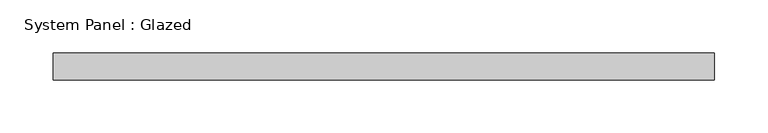
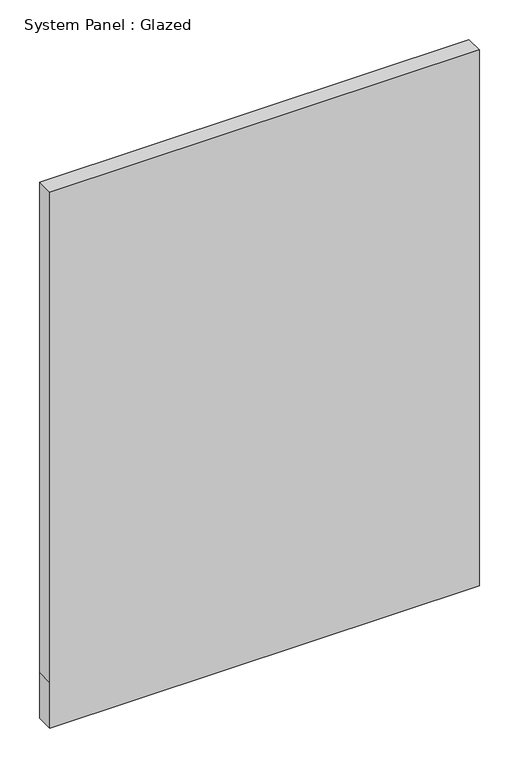
"""IFC4 building model written with IfcOpenShell, lengths in millimetres: plate geometry, System Panel : Glazed."""

from ifc_helpers import new_model, si_unit, frame, origin, place, context, project, spatial, polyline, outline, extrude, source, transform, mapped, element, save


def system_panel_glazed_6c4ef35e(model_context):
    return source(origin(), model_context, "Body", "SweptSolid", [
        extrude(outline(polyline([(0.0, -311.15), (0.0, 311.15), (69.85, 311.15), (820.9261324, 311.15), (820.9261324, -311.15), (69.85, -311.15), (0.0, -311.15)])), frame((0.0, 19.05, 0.0), z_axis=(0.0, 1.0, 0.0), x_axis=(0.0, 0.0, 1.0)), (0.0, 0.0, 1.0), 25.4),
    ])


if __name__ == "__main__":
    model = new_model("IFC4")
    model_context = context("Model", 3, world=origin())
    ifc_project = project(units=[si_unit("LENGTHUNIT", "METRE", prefix="MILLI")], contexts=[model_context])
    site = spatial("IfcSite", under=ifc_project)
    building = spatial("IfcBuilding", under=site)
    placement = place(None, origin())
    system_panel_glazed_shape = system_panel_glazed_6c4ef35e(model_context)
    element("IfcPlate", 1, ObjectType="System Panel : Glazed", at=placement, inside=building, context=model_context, shape_type="MappedRepresentation", body=[
        mapped(system_panel_glazed_shape, transform((0.0, 0.0, 0.0), x_axis=(1.0, 0.0, 0.0), y_axis=(0.0, 1.0, 0.0), z_axis=(0.0, 0.0, 1.0))),
    ])
    save(model, "model.ifc")

# Revit data of these elements
# Type "System Panel : Glazed"
#   Construction Type Id = "GSP4R"
#   Analytic Construction = "1/8 in Pilkington single glazing"
#   Visual Light Transmittance = 0.9
#   Solar Heat Gain Coefficient = 0.86
#   Heat Transfer Coefficient (U) = 1.18115 BTU/(h·ft²·°F)
#   Define Thermal Properties by = 1
# Element 1 (IfcPlate, "System Panel : Glazed")
#   Materials on its faces: "Glass"
# Materials
#   "Glass": class "Glass", colour RGB 0 128 192, transparency 0.75, Description = "Soda Lime Glass", Cost = 0
